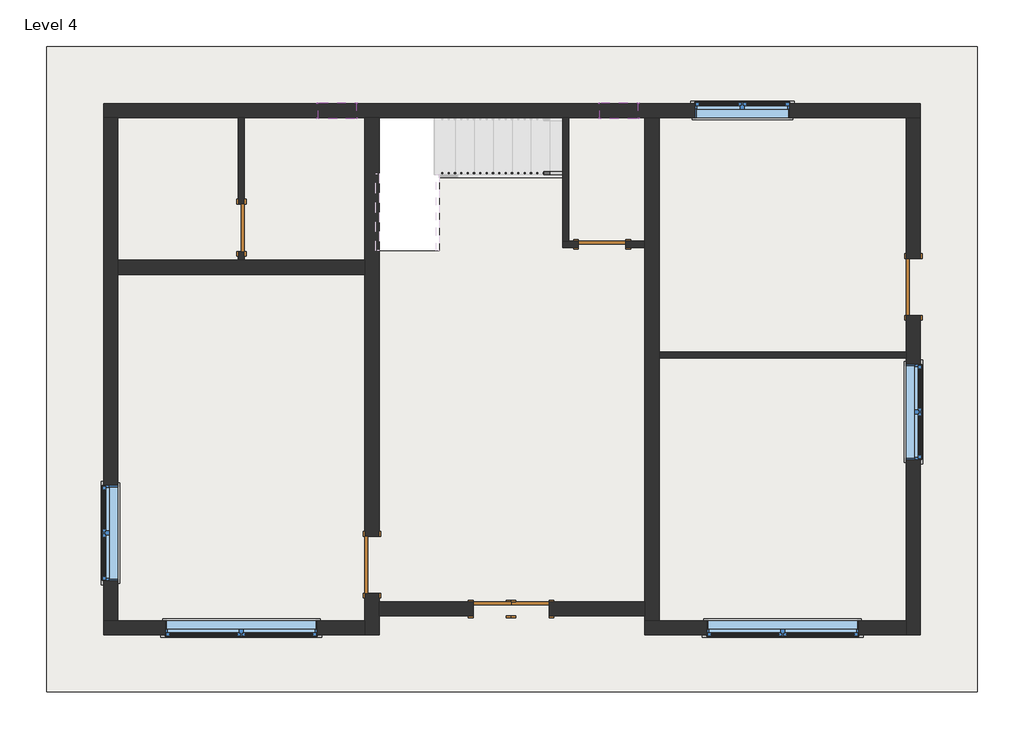
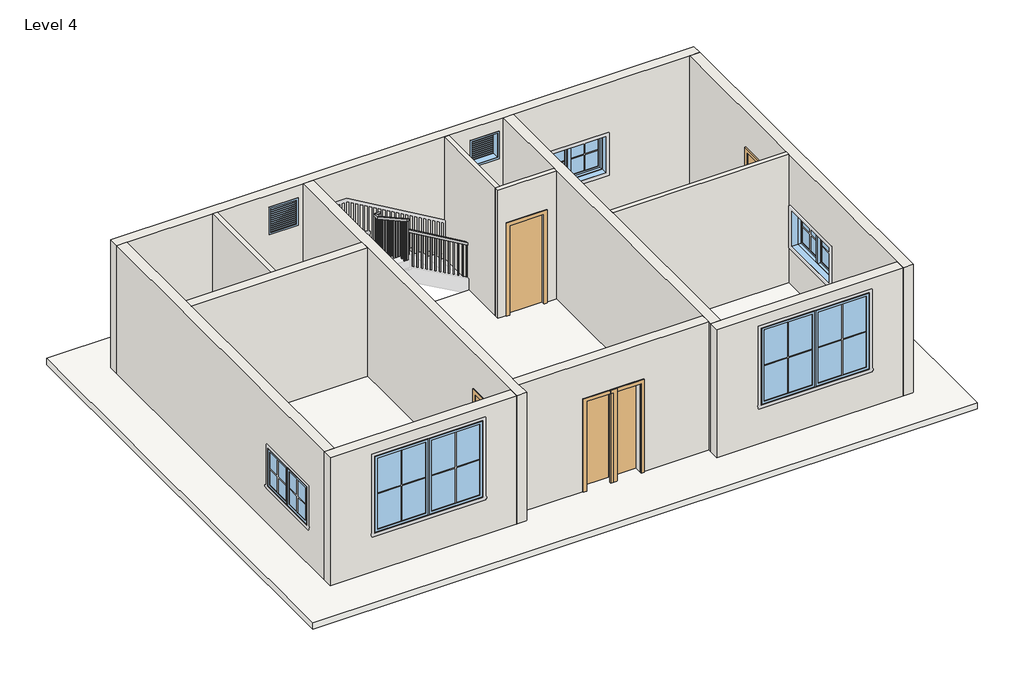
# One storey, part 1 of 2: 13 walls, 7 windows, 6 doors, 1 railing, 1 roof.
"""IFC4 building model written with IfcOpenShell, lengths in millimetres."""

from ifc_helpers import new_model, si_unit, frame, origin, place, context, project, spatial, polyline, outline, extrude, faceted_brep, transform, mapped, element, save
from components import single_flush_door_2_4a3212df, single_flush_door_2_0d3b4037, door_270f2424, door_aa9e95e7, single_flush_door_3_a90ba1ad, window_casement_double_c1d95f0f, window_casement_double_9ae172a2, window_f2d8fef0

model = new_model("IFC4")

# Units and contexts
model_context = context("Model", 3, world=origin())
ifc_project = project(units=[si_unit("LENGTHUNIT", "METRE", prefix="MILLI")], contexts=[model_context])

# Site, building, storey
site = spatial("IfcSite", under=ifc_project)
building = spatial("IfcBuilding", under=site)
storey = spatial("IfcBuildingStorey", under=building, Name="Level 4", Elevation=9448.8)

# Doors
placement = place(None, origin())
single_flush_door_2_shape = single_flush_door_2_4a3212df(model_context)
element("IfcDoor", 1, ObjectType="Single-Flush : DOOR 2'", at=placement, inside=storey, context=model_context, shape_type="MappedRepresentation", body=[
    mapped(single_flush_door_2_shape, transform((-1572.7415084, -2604.3618005, 9448.8), x_axis=(-1.0, 0.0, 0.0), y_axis=(0.0, -1.0, 0.0), z_axis=(0.0, 0.0, 1.0))),
])
single_flush_door_2_2_shape = single_flush_door_2_0d3b4037(model_context)
element("IfcDoor", 2, ObjectType="Single-Flush : DOOR 2'", at=placement, inside=storey, context=model_context, shape_type="MappedRepresentation", body=[
    mapped(single_flush_door_2_2_shape, transform((-963.1415084, -2604.3618005, 9448.8), x_axis=(1.0, 0.0, 0.0), y_axis=(0.0, 1.0, 0.0), z_axis=(0.0, 0.0, 1.0))),
])
door_shape = door_270f2424(model_context)
element("IfcDoor", 3, ObjectType="Single-Flush : DOOR 2'6\"", at=placement, inside=storey, context=model_context, shape_type="MappedRepresentation", body=[
    mapped(door_shape, transform((-5598.6415084, 3517.0381995, 9448.8), x_axis=(0.0, -1.0, 0.0), y_axis=(1.0, 0.0, 0.0), z_axis=(0.0, 0.0, 1.0))),
])
door_2_shape = door_aa9e95e7(model_context)
element("IfcDoor", 4, ObjectType="Single-Flush : DOOR 2'6\"", at=placement, inside=storey, context=model_context, shape_type="MappedRepresentation", body=[
    mapped(door_2_shape, transform((192.5584916, 3250.3381995, 9448.8), x_axis=(-1.0, 0.0, 0.0), y_axis=(0.0, -1.0, 0.0), z_axis=(0.0, 0.0, 1.0))),
])
single_flush_door_3_shape = single_flush_door_3_a90ba1ad(model_context)
element("IfcDoor", 5, ObjectType="Single-Flush : DOOR 3'", at=placement, inside=storey, context=model_context, shape_type="MappedRepresentation", body=[
    mapped(single_flush_door_3_shape, transform((-3503.1415084, -1893.1618005, 9448.8), x_axis=(0.0, -1.0, 0.0), y_axis=(1.0, 0.0, 0.0), z_axis=(0.0, 0.0, 1.0))),
])
element("IfcDoor", 6, ObjectType="Single-Flush : DOOR 3'", at=placement, inside=storey, context=model_context, shape_type="MappedRepresentation", body=[
    mapped(single_flush_door_3_shape, transform((5183.6584916, 2564.5381995, 9448.8), x_axis=(0.0, -1.0, 0.0), y_axis=(1.0, 0.0, 0.0), z_axis=(0.0, 0.0, 1.0))),
])

# Railing
element("IfcRailing", 7, ObjectType="Handrail - Rectangular", at=placement, inside=storey, context=model_context, shape_type="SolidModel", body=[
    faceted_brep([(-442.4415084, 4368.3146777, 10532.5333333), (-442.4415084, 4368.3146777, 10473.7219871), (-442.4415084, 4419.1146777, 10473.7219871), (-442.4415084, 4419.1146777, 10532.5333333), (-2398.2415084, 4368.3146777, 11673.4166667), (-2449.0415084, 4368.3146777, 11644.2386538), (-2449.0415084, 4419.1146777, 11644.2386538), (-2398.2415084, 4419.1146777, 11673.4166667), (-2398.2415084, 4368.3146777, 11929.5202697), (-2449.0415084, 4368.3146777, 11878.7202697), (-2449.0415084, 4419.1146777, 11878.7202697), (-2398.2415084, 4419.1146777, 11929.5202697), (-2474.4415084, 4368.3146777, 11929.5202697), (-2474.4415084, 4368.3146777, 11878.7202697), (-2525.2415084, 4419.1146777, 11878.7202697), (-2525.2415084, 4419.1146777, 11929.5202697), (-2474.4415084, 4292.1146777, 11929.5202697), (-2474.4415084, 4278.9546266, 11878.7202697), (-2525.2415084, 4278.9546266, 11878.7202697), (-2525.2415084, 4292.1146777, 11929.5202697), (-2474.4415084, 3148.7383287, 12564.5333333), (-2525.2415084, 3148.7383287, 12564.5333333), (-2525.2415084, 3148.7383287, 12506.42445), (-2474.4415084, 3148.7383287, 12506.42445)], [[[0, 1, 2, 3]], [[1, 0, 4, 5]], [[2, 1, 5, 6]], [[3, 2, 6, 7]], [[0, 3, 7, 4]], [[5, 4, 8, 9]], [[6, 5, 9, 10]], [[7, 6, 10, 11]], [[4, 7, 11, 8]], [[9, 8, 12, 13]], [[10, 9, 13, 14]], [[11, 10, 14, 15]], [[8, 11, 15, 12]], [[13, 12, 16, 17]], [[14, 13, 17, 18]], [[15, 14, 18, 19]], [[12, 15, 19, 16]], [[20, 21, 22, 23]], [[17, 16, 20, 23]], [[18, 17, 23, 22]], [[19, 18, 22, 21]], [[16, 19, 21, 20]]]),
    extrude(outline(polyline([(3184.0396777, 12486.9754052), (3184.0396777, 11480.8), (3164.9896777, 11480.8), (3164.9896777, 12497.5554726), (3184.0396777, 12486.9754052)])), frame((-2509.3665084, 0.0, 0.0), z_axis=(1.0, 0.0, 0.0), x_axis=(0.0, 1.0, 0.0)), (0.0, 0.0, 1.0), 19.05),
    extrude(outline(polyline([(3285.6396777, 12430.5483789), (3285.6396777, 11480.8), (3266.5896777, 11480.8), (3266.5896777, 12441.1284463), (3285.6396777, 12430.5483789)])), frame((-2509.3665084, 0.0, 0.0), z_axis=(1.0, 0.0, 0.0), x_axis=(0.0, 1.0, 0.0)), (0.0, 0.0, 1.0), 19.05),
    extrude(outline(polyline([(3387.2396777, 12374.1213526), (3387.2396777, 11480.8), (3368.1896777, 11480.8), (3368.1896777, 12384.7014201), (3387.2396777, 12374.1213526)])), frame((-2509.3665084, 0.0, 0.0), z_axis=(1.0, 0.0, 0.0), x_axis=(0.0, 1.0, 0.0)), (0.0, 0.0, 1.0), 19.05),
    extrude(outline(polyline([(3488.8396777, 12317.6420718), (3488.8396777, 11311.4666667), (3469.7896777, 11311.4666667), (3469.7896777, 12328.2221392), (3488.8396777, 12317.6420718)])), frame((-2509.3665084, 0.0, 0.0), z_axis=(1.0, 0.0, 0.0), x_axis=(0.0, 1.0, 0.0)), (0.0, 0.0, 1.0), 19.05),
    extrude(outline(polyline([(3590.4396777, 12261.2150456), (3590.4396777, 11311.4666667), (3571.3896777, 11311.4666667), (3571.3896777, 12271.795113), (3590.4396777, 12261.2150456)])), frame((-2509.3665084, 0.0, 0.0), z_axis=(1.0, 0.0, 0.0), x_axis=(0.0, 1.0, 0.0)), (0.0, 0.0, 1.0), 19.05),
    extrude(outline(polyline([(3692.0396777, 12204.7880193), (3692.0396777, 11311.4666667), (3672.9896777, 11311.4666667), (3672.9896777, 12215.3680867), (3692.0396777, 12204.7880193)])), frame((-2509.3665084, 0.0, 0.0), z_axis=(1.0, 0.0, 0.0), x_axis=(0.0, 1.0, 0.0)), (0.0, 0.0, 1.0), 19.05),
    extrude(outline(polyline([(3793.6396777, 12148.3087385), (3793.6396777, 11142.1333333), (3774.5896777, 11142.1333333), (3774.5896777, 12158.8888059), (3793.6396777, 12148.3087385)])), frame((-2509.3665084, 0.0, 0.0), z_axis=(1.0, 0.0, 0.0), x_axis=(0.0, 1.0, 0.0)), (0.0, 0.0, 1.0), 19.05),
    extrude(outline(polyline([(3895.2396777, 12091.8817122), (3895.2396777, 11142.1333333), (3876.1896777, 11142.1333333), (3876.1896777, 12102.4617797), (3895.2396777, 12091.8817122)])), frame((-2509.3665084, 0.0, 0.0), z_axis=(1.0, 0.0, 0.0), x_axis=(0.0, 1.0, 0.0)), (0.0, 0.0, 1.0), 19.05),
    extrude(outline(polyline([(3996.8396777, 12035.454686), (3996.8396777, 11142.1333333), (3977.7896777, 11142.1333333), (3977.7896777, 12046.0347534), (3996.8396777, 12035.454686)])), frame((-2509.3665084, 0.0, 0.0), z_axis=(1.0, 0.0, 0.0), x_axis=(0.0, 1.0, 0.0)), (0.0, 0.0, 1.0), 19.05),
    extrude(outline(polyline([(4098.4396777, 11978.9754052), (4098.4396777, 10972.8), (4079.3896777, 10972.8), (4079.3896777, 11989.5554726), (4098.4396777, 11978.9754052)])), frame((-2509.3665084, 0.0, 0.0), z_axis=(1.0, 0.0, 0.0), x_axis=(0.0, 1.0, 0.0)), (0.0, 0.0, 1.0), 19.05),
    extrude(outline(polyline([(4200.0396777, 11922.5483789), (4200.0396777, 10972.8), (4180.9896777, 10972.8), (4180.9896777, 11933.1284463), (4200.0396777, 11922.5483789)])), frame((-2509.3665084, 0.0, 0.0), z_axis=(1.0, 0.0, 0.0), x_axis=(0.0, 1.0, 0.0)), (0.0, 0.0, 1.0), 19.05),
    extrude(outline(polyline([(4301.6396777, 11866.1213526), (4301.6396777, 10972.8), (4282.5896777, 10972.8), (4282.5896777, 11876.7014201), (4301.6396777, 11866.1213526)])), frame((-2509.3665084, 0.0, 0.0), z_axis=(1.0, 0.0, 0.0), x_axis=(0.0, 1.0, 0.0)), (0.0, 0.0, 1.0), 19.05),
    extrude(outline(polyline([(-2464.9165084, 4384.1896777), (-2483.9665084, 4384.1896777), (-2483.9665084, 4403.2396777), (-2464.9165084, 4403.2396777), (-2464.9165084, 4384.1896777)])), frame((0.0, 0.0, 10803.4666667), z_axis=(0.0, 0.0, 1.0), x_axis=(1.0, 0.0, 0.0)), (0.0, 0.0, 1.0), 1075.253603),
    extrude(outline(polyline([(11605.3449038, -2382.3665084), (10634.1333333, -2382.3665084), (10634.1333333, -2363.3165084), (11594.2324038, -2363.3165084), (11605.3449038, -2382.3665084)])), frame((0.0, 4384.1896777, 0.0), z_axis=(0.0, 1.0, 0.0), x_axis=(0.0, 0.0, 1.0)), (0.0, 0.0, 1.0), 19.05),
    extrude(outline(polyline([(11546.0782371, -2280.7665084), (10634.1333333, -2280.7665084), (10634.1333333, -2261.7165084), (11534.9657371, -2261.7165084), (11546.0782371, -2280.7665084)])), frame((0.0, 4384.1896777, 0.0), z_axis=(0.0, 1.0, 0.0), x_axis=(0.0, 0.0, 1.0)), (0.0, 0.0, 1.0), 19.05),
    extrude(outline(polyline([(11486.8115704, -2179.1665084), (10634.1333333, -2179.1665084), (10634.1333333, -2160.1165084), (11475.6990704, -2160.1165084), (11486.8115704, -2179.1665084)])), frame((0.0, 4384.1896777, 0.0), z_axis=(0.0, 1.0, 0.0), x_axis=(0.0, 0.0, 1.0)), (0.0, 0.0, 1.0), 19.05),
    extrude(outline(polyline([(11427.5449038, -2077.5665084), (10464.8, -2077.5665084), (10464.8, -2058.5165084), (11416.4324038, -2058.5165084), (11427.5449038, -2077.5665084)])), frame((0.0, 4384.1896777, 0.0), z_axis=(0.0, 1.0, 0.0), x_axis=(0.0, 0.0, 1.0)), (0.0, 0.0, 1.0), 19.05),
    extrude(outline(polyline([(11368.2782371, -1975.9665084), (10464.8, -1975.9665084), (10464.8, -1956.9165084), (11357.1657371, -1956.9165084), (11368.2782371, -1975.9665084)])), frame((0.0, 4384.1896777, 0.0), z_axis=(0.0, 1.0, 0.0), x_axis=(0.0, 0.0, 1.0)), (0.0, 0.0, 1.0), 19.05),
    extrude(outline(polyline([(11309.0115704, -1874.3665084), (10464.8, -1874.3665084), (10464.8, -1855.3165084), (11297.8990704, -1855.3165084), (11309.0115704, -1874.3665084)])), frame((0.0, 4384.1896777, 0.0), z_axis=(0.0, 1.0, 0.0), x_axis=(0.0, 0.0, 1.0)), (0.0, 0.0, 1.0), 19.05),
    extrude(outline(polyline([(11249.7449038, -1772.7665084), (10295.4666667, -1772.7665084), (10295.4666667, -1753.7165084), (11238.6324038, -1753.7165084), (11249.7449038, -1772.7665084)])), frame((0.0, 4384.1896777, 0.0), z_axis=(0.0, 1.0, 0.0), x_axis=(0.0, 0.0, 1.0)), (0.0, 0.0, 1.0), 19.05),
    extrude(outline(polyline([(11190.4782371, -1671.1665084), (10295.4666667, -1671.1665084), (10295.4666667, -1652.1165084), (11179.3657371, -1652.1165084), (11190.4782371, -1671.1665084)])), frame((0.0, 4384.1896777, 0.0), z_axis=(0.0, 1.0, 0.0), x_axis=(0.0, 0.0, 1.0)), (0.0, 0.0, 1.0), 19.05),
    extrude(outline(polyline([(11131.2115704, -1569.5665084), (10295.4666667, -1569.5665084), (10295.4666667, -1550.5165084), (11120.0990704, -1550.5165084), (11131.2115704, -1569.5665084)])), frame((0.0, 4384.1896777, 0.0), z_axis=(0.0, 1.0, 0.0), x_axis=(0.0, 0.0, 1.0)), (0.0, 0.0, 1.0), 19.05),
    extrude(outline(polyline([(11071.9449038, -1467.9665084), (10126.1333333, -1467.9665084), (10126.1333333, -1448.9165084), (11060.8324038, -1448.9165084), (11071.9449038, -1467.9665084)])), frame((0.0, 4384.1896777, 0.0), z_axis=(0.0, 1.0, 0.0), x_axis=(0.0, 0.0, 1.0)), (0.0, 0.0, 1.0), 19.05),
    extrude(outline(polyline([(11012.6782371, -1366.3665084), (10126.1333333, -1366.3665084), (10126.1333333, -1347.3165084), (11001.5657371, -1347.3165084), (11012.6782371, -1366.3665084)])), frame((0.0, 4384.1896777, 0.0), z_axis=(0.0, 1.0, 0.0), x_axis=(0.0, 0.0, 1.0)), (0.0, 0.0, 1.0), 19.05),
    extrude(outline(polyline([(10953.4115704, -1264.7665084), (10126.1333333, -1264.7665084), (10126.1333333, -1245.7165084), (10942.2990704, -1245.7165084), (10953.4115704, -1264.7665084)])), frame((0.0, 4384.1896777, 0.0), z_axis=(0.0, 1.0, 0.0), x_axis=(0.0, 0.0, 1.0)), (0.0, 0.0, 1.0), 19.05),
    extrude(outline(polyline([(10894.1449038, -1163.1665084), (9956.8, -1163.1665084), (9956.8, -1144.1165084), (10883.0324038, -1144.1165084), (10894.1449038, -1163.1665084)])), frame((0.0, 4384.1896777, 0.0), z_axis=(0.0, 1.0, 0.0), x_axis=(0.0, 0.0, 1.0)), (0.0, 0.0, 1.0), 19.05),
    extrude(outline(polyline([(10834.8782371, -1061.5665084), (9956.8, -1061.5665084), (9956.8, -1042.5165084), (10823.7657371, -1042.5165084), (10834.8782371, -1061.5665084)])), frame((0.0, 4384.1896777, 0.0), z_axis=(0.0, 1.0, 0.0), x_axis=(0.0, 0.0, 1.0)), (0.0, 0.0, 1.0), 19.05),
    extrude(outline(polyline([(10775.6115704, -959.9665084), (9956.8, -959.9665084), (9956.8, -940.9165084), (10764.4990704, -940.9165084), (10775.6115704, -959.9665084)])), frame((0.0, 4384.1896777, 0.0), z_axis=(0.0, 1.0, 0.0), x_axis=(0.0, 0.0, 1.0)), (0.0, 0.0, 1.0), 19.05),
    extrude(outline(polyline([(10716.3449038, -858.3665084), (9787.4666667, -858.3665084), (9787.4666667, -839.3165084), (10705.2324038, -839.3165084), (10716.3449038, -858.3665084)])), frame((0.0, 4384.1896777, 0.0), z_axis=(0.0, 1.0, 0.0), x_axis=(0.0, 0.0, 1.0)), (0.0, 0.0, 1.0), 19.05),
    extrude(outline(polyline([(10657.0782371, -756.7665084), (9787.4666667, -756.7665084), (9787.4666667, -737.7165084), (10645.9657371, -737.7165084), (10657.0782371, -756.7665084)])), frame((0.0, 4384.1896777, 0.0), z_axis=(0.0, 1.0, 0.0), x_axis=(0.0, 0.0, 1.0)), (0.0, 0.0, 1.0), 19.05),
    extrude(outline(polyline([(10597.8115704, -655.1665084), (9787.4666667, -655.1665084), (9787.4666667, -636.1165084), (10586.6990704, -636.1165084), (10597.8115704, -655.1665084)])), frame((0.0, 4384.1896777, 0.0), z_axis=(0.0, 1.0, 0.0), x_axis=(0.0, 0.0, 1.0)), (0.0, 0.0, 1.0), 19.05),
    extrude(outline(polyline([(10538.5449038, -553.5665084), (9618.1333333, -553.5665084), (9618.1333333, -534.5165084), (10527.4324038, -534.5165084), (10538.5449038, -553.5665084)])), frame((0.0, 4384.1896777, 0.0), z_axis=(0.0, 1.0, 0.0), x_axis=(0.0, 0.0, 1.0)), (0.0, 0.0, 1.0), 19.05),
    extrude(outline(polyline([(-2490.3165084, 4384.1896777), (-2509.3665084, 4384.1896777), (-2509.3665084, 4403.2396777), (-2490.3165084, 4403.2396777), (-2490.3165084, 4384.1896777)])), frame((0.0, 0.0, 10803.4666667), z_axis=(0.0, 0.0, 1.0), x_axis=(1.0, 0.0, 0.0)), (0.0, 0.0, 1.0), 1075.253603),
    extrude(outline(polyline([(3167.7883287, 12495.8443826), (3167.7883287, 11480.8), (3148.7383287, 11480.8), (3148.7383287, 12506.42445), (3167.7883287, 12495.8443826)])), frame((-2509.3665084, 0.0, 0.0), z_axis=(1.0, 0.0, 0.0), x_axis=(0.0, 1.0, 0.0)), (0.0, 0.0, 1.0), 19.05),
    extrude(outline(polyline([(10484.8344871, -461.4915084), (9618.1333333, -461.4915084), (9618.1333333, -442.4415084), (10473.7219871, -442.4415084), (10484.8344871, -461.4915084)])), frame((0.0, 4384.1896777, 0.0), z_axis=(0.0, 1.0, 0.0), x_axis=(0.0, 0.0, 1.0)), (0.0, 0.0, 1.0), 19.05),
])

# Roof
element("IfcRoof", 8, ObjectType="ROOF 6\"", at=placement, inside=storey, context=model_context, shape_type="SweptSolid", body=[
    extrude(outline(polyline([(-8722.8415084, -3937.8618005), (-8722.8415084, 6425.3381995), (6212.3584916, 6425.3381995), (6212.3584916, -3937.8618005), (-8722.8415084, -3937.8618005)]), holes=[polyline([(-3439.6415084, 5333.1381995), (-3439.6415084, 3148.7383287), (-2423.6415084, 3148.7383287), (-2423.6415084, 4317.5146777), (-442.4415084, 4317.5146777), (-442.4415084, 5333.1381995), (-3439.6415084, 5333.1381995)])]), frame((0.0, 0.0, 9296.4), z_axis=(0.0, 0.0, 1.0), x_axis=(1.0, 0.0, 0.0)), (0.0, 0.0, 1.0), 152.4),
])

# Walls
element("IfcWall", 9, ObjectType="WALL 4\"", at=placement, inside=storey, context=model_context, shape_type="SweptSolid", body=[
    extrude(outline(polyline([(3136.0381995, 11582.4), (3136.0381995, 9448.8), (2996.3381995, 9448.8), (2996.3381995, 12496.8), (5282.3381995, 12496.8), (5282.3381995, 9448.8), (3898.0381995, 9448.8), (3898.0381995, 11582.4), (3136.0381995, 11582.4)])), frame((-5649.4415084, 0.0, 0.0), z_axis=(1.0, 0.0, 0.0), x_axis=(0.0, 1.0, 0.0)), (0.0, 0.0, 1.0), 101.6),
])
element("IfcWall", 10, ObjectType="WALL 4\"", at=placement, inside=storey, context=model_context, shape_type="Brep", body=[
    faceted_brep([(-188.4415084, 3301.1381995, 11582.4), (-188.4415084, 3301.1381995, 9448.8), (-340.8415084, 3301.1381995, 9448.8), (-442.4415084, 3301.1381995, 9448.8), (-442.4415084, 3301.1381995, 12496.8), (-340.8415084, 3301.1381995, 12496.8), (878.3584916, 3301.1381995, 12496.8), (878.3584916, 3301.1381995, 9448.8), (573.5584916, 3301.1381995, 9448.8), (573.5584916, 3301.1381995, 11582.4), (-442.4415084, 3199.5381995, 9448.8), (-188.4415084, 3199.5381995, 9448.8), (-188.4415084, 3199.5381995, 11582.4), (573.5584916, 3199.5381995, 11582.4), (573.5584916, 3199.5381995, 9448.8), (878.3584916, 3199.5381995, 9448.8), (878.3584916, 3199.5381995, 12496.8), (-442.4415084, 3199.5381995, 12496.8)], [[[0, 1, 2, 3, 4, 5, 6, 7, 8, 9]], [[10, 11, 12, 13, 14, 15, 16, 17]], [[8, 7, 15, 14]], [[3, 2, 1, 11, 10]], [[7, 6, 16, 15]], [[4, 3, 10, 17]], [[12, 11, 1, 0]], [[13, 12, 0, 9]], [[14, 13, 9, 8]], [[6, 5, 4, 17, 16]]]),
])
element("IfcWall", 11, ObjectType="WALL 4\"", at=placement, inside=storey, context=model_context, shape_type="Brep", body=[
    faceted_brep([(-340.8415084, 3301.1381995, 9448.8), (-340.8415084, 5282.3381995, 9448.8), (-340.8415084, 5282.3381995, 12496.8), (-340.8415084, 3301.1381995, 12496.8), (-442.4415084, 3301.1381995, 9448.8), (-442.4415084, 3301.1381995, 12496.8), (-442.4415084, 4317.5146777, 12496.8), (-442.4415084, 5282.3381995, 12496.8), (-442.4415084, 5282.3381995, 9448.8)], [[[0, 1, 2, 3]], [[4, 5, 6, 7, 8]], [[1, 0, 4, 8]], [[0, 3, 5, 4]], [[2, 1, 8, 7]], [[3, 2, 7, 6, 5]]]),
])
element("IfcWall", 12, ObjectType="WALL 4\"", at=placement, inside=storey, context=model_context, shape_type="SweptSolid", body=[
    extrude(outline(polyline([(1106.9584916, 1523.1381995), (5069.3584916, 1523.1381995), (5069.3584916, 1421.5381995), (1106.9584916, 1421.5381995), (1106.9584916, 1523.1381995)])), frame((0.0, 0.0, 9448.8), z_axis=(0.0, 0.0, 1.0), x_axis=(1.0, 0.0, 0.0)), (0.0, 0.0, 1.0), 3048.0),
])
element("IfcWall", 13, ObjectType="WALL 9\"", at=placement, inside=storey, context=model_context, shape_type="Brep", body=[
    faceted_brep([(-7808.4415084, 5282.3381995, 9448.8), (-7579.8415084, 5282.3381995, 9448.8), (-5649.4415084, 5282.3381995, 9448.8), (-5547.8415084, 5282.3381995, 9448.8), (-3617.4415084, 5282.3381995, 9448.8), (-3388.8415084, 5282.3381995, 9448.8), (-442.4415084, 5282.3381995, 9448.8), (-340.8415084, 5282.3381995, 9448.8), (878.3584916, 5282.3381995, 9448.8), (1106.9584916, 5282.3381995, 9448.8), (5069.3584916, 5282.3381995, 9448.8), (5297.9584916, 5282.3381995, 9448.8), (5297.9584916, 5282.3381995, 12496.8), (5069.3584916, 5282.3381995, 12496.8), (1106.9584916, 5282.3381995, 12496.8), (878.3584916, 5282.3381995, 12496.8), (-340.8415084, 5282.3381995, 12496.8), (-442.4415084, 5282.3381995, 12496.8), (-3388.8415084, 5282.3381995, 12496.8), (-3617.4415084, 5282.3381995, 12496.8), (-5547.8415084, 5282.3381995, 12496.8), (-5649.4415084, 5282.3381995, 12496.8), (-7579.8415084, 5282.3381995, 12496.8), (-7808.4415084, 5282.3381995, 12496.8), (3202.4584916, 5282.3381995, 11277.6), (3202.4584916, 5282.3381995, 10363.2), (1678.4584916, 5282.3381995, 10363.2), (1678.4584916, 5282.3381995, 11277.6), (154.4584916, 5282.3381995, 12192.0), (764.0584916, 5282.3381995, 12192.0), (764.0584916, 5282.3381995, 11582.4), (154.4584916, 5282.3381995, 11582.4), (-3757.1415084, 5282.3381995, 12192.0), (-3757.1415084, 5282.3381995, 11582.4), (-4366.7415084, 5282.3381995, 11582.4), (-4366.7415084, 5282.3381995, 12192.0), (-7808.4415084, 5510.9381995, 9448.8), (-7808.4415084, 5510.9381995, 12496.8), (5297.9584916, 5510.9381995, 12496.8), (5297.9584916, 5510.9381995, 9448.8), (3202.4584916, 5510.9381995, 11277.6), (1678.4584916, 5510.9381995, 11277.6), (1678.4584916, 5510.9381995, 10363.2), (3202.4584916, 5510.9381995, 10363.2), (154.4584916, 5510.9381995, 12192.0), (154.4584916, 5510.9381995, 11582.4), (764.0584916, 5510.9381995, 11582.4), (764.0584916, 5510.9381995, 12192.0), (-3757.1415084, 5510.9381995, 12192.0), (-4366.7415084, 5510.9381995, 12192.0), (-4366.7415084, 5510.9381995, 11582.4), (-3757.1415084, 5510.9381995, 11582.4)], [[[0, 1, 2, 3, 4, 5, 6, 7, 8, 9, 10, 11, 12, 13, 14, 15, 16, 17, 18, 19, 20, 21, 22, 23], [24, 25, 26, 27], [28, 29, 30, 31], [32, 33, 34, 35]], [[36, 37, 38, 39], [40, 41, 42, 43], [44, 45, 46, 47], [48, 49, 50, 51]], [[11, 10, 9, 8, 7, 6, 5, 4, 3, 2, 1, 0, 36, 39]], [[23, 22, 21, 20, 19, 18, 17, 16, 15, 14, 13, 12, 38, 37]], [[12, 11, 39, 38]], [[0, 23, 37, 36]], [[25, 24, 40, 43]], [[26, 25, 43, 42]], [[27, 26, 42, 41]], [[24, 27, 41, 40]], [[45, 44, 28, 31]], [[46, 45, 31, 30]], [[47, 46, 30, 29]], [[44, 47, 29, 28]], [[33, 32, 48, 51]], [[34, 33, 51, 50]], [[35, 34, 50, 49]], [[32, 35, 49, 48]]]),
])
element("IfcWall", 14, ObjectType="WALL 9\"", at=placement, inside=storey, context=model_context, shape_type="Brep", body=[
    faceted_brep([(5069.3584916, 2107.3381995, 11582.4), (5069.3584916, 2107.3381995, 9448.8), (5069.3584916, 1523.1381995, 9448.8), (5069.3584916, 1421.5381995, 9448.8), (5069.3584916, -2794.8618005, 9448.8), (5069.3584916, -3023.4618005, 9448.8), (5069.3584916, -3023.4618005, 12496.8), (5069.3584916, -2794.8618005, 12496.8), (5069.3584916, 1421.5381995, 12496.8), (5069.3584916, 1523.1381995, 12496.8), (5069.3584916, 5282.3381995, 12496.8), (5069.3584916, 5282.3381995, 9448.8), (5069.3584916, 3021.7381995, 9448.8), (5069.3584916, 3021.7381995, 11582.4), (5069.3584916, -204.0618005, 11277.6), (5069.3584916, -204.0618005, 10363.2), (5069.3584916, 1319.9381995, 10363.2), (5069.3584916, 1319.9381995, 11277.6), (5297.9584916, -3023.4618005, 9448.8), (5297.9584916, 2107.3381995, 9448.8), (5297.9584916, 2107.3381995, 11582.4), (5297.9584916, 3021.7381995, 11582.4), (5297.9584916, 3021.7381995, 9448.8), (5297.9584916, 5282.3381995, 9448.8), (5297.9584916, 5282.3381995, 12496.8), (5297.9584916, -3023.4618005, 12496.8), (5297.9584916, -204.0618005, 11277.6), (5297.9584916, 1319.9381995, 11277.6), (5297.9584916, 1319.9381995, 10363.2), (5297.9584916, -204.0618005, 10363.2)], [[[0, 1, 2, 3, 4, 5, 6, 7, 8, 9, 10, 11, 12, 13], [14, 15, 16, 17]], [[18, 19, 20, 21, 22, 23, 24, 25], [26, 27, 28, 29]], [[12, 11, 23, 22]], [[5, 4, 3, 2, 1, 19, 18]], [[11, 10, 24, 23]], [[6, 5, 18, 25]], [[15, 14, 26, 29]], [[16, 15, 29, 28]], [[17, 16, 28, 27]], [[14, 17, 27, 26]], [[20, 19, 1, 0]], [[21, 20, 0, 13]], [[22, 21, 13, 12]], [[10, 9, 8, 7, 6, 25, 24]]]),
])
element("IfcWall", 15, ObjectType="WALL 9\"", at=placement, inside=storey, context=model_context, shape_type="Brep", body=[
    faceted_brep([(5069.3584916, -2794.8618005, 9448.8), (1106.9584916, -2794.8618005, 9448.8), (878.3584916, -2794.8618005, 9448.8), (878.3584916, -2794.8618005, 12496.8), (1106.9584916, -2794.8618005, 12496.8), (5069.3584916, -2794.8618005, 12496.8), (1868.9584916, -2794.8618005, 12192.0), (1868.9584916, -2794.8618005, 10363.2), (4307.3584916, -2794.8618005, 10363.2), (4307.3584916, -2794.8618005, 12192.0), (5069.3584916, -3023.4618005, 9448.8), (5069.3584916, -3023.4618005, 12496.8), (878.3584916, -3023.4618005, 12496.8), (878.3584916, -3023.4618005, 9448.8), (1868.9584916, -3023.4618005, 12192.0), (4307.3584916, -3023.4618005, 12192.0), (4307.3584916, -3023.4618005, 10363.2), (1868.9584916, -3023.4618005, 10363.2)], [[[0, 1, 2, 3, 4, 5], [6, 7, 8, 9]], [[10, 11, 12, 13], [14, 15, 16, 17]], [[2, 1, 0, 10, 13]], [[0, 5, 11, 10]], [[3, 2, 13, 12]], [[7, 6, 14, 17]], [[8, 7, 17, 16]], [[9, 8, 16, 15]], [[6, 9, 15, 14]], [[5, 4, 3, 12, 11]]]),
])
element("IfcWall", 16, ObjectType="WALL 9\"", at=placement, inside=storey, context=model_context, shape_type="Brep", body=[
    faceted_brep([(1106.9584916, -2794.8618005, 9448.8), (1106.9584916, 1421.5381995, 9448.8), (1106.9584916, 1523.1381995, 9448.8), (1106.9584916, 5282.3381995, 9448.8), (1106.9584916, 5282.3381995, 12496.8), (1106.9584916, 1523.1381995, 12496.8), (1106.9584916, 1421.5381995, 12496.8), (1106.9584916, -2794.8618005, 12496.8), (878.3584916, -2794.8618005, 9448.8), (878.3584916, -2794.8618005, 12496.8), (878.3584916, -2718.6618005, 12496.8), (878.3584916, -2490.0618005, 12496.8), (878.3584916, 3199.5381995, 12496.8), (878.3584916, 3301.1381995, 12496.8), (878.3584916, 5282.3381995, 12496.8), (878.3584916, 5282.3381995, 9448.8), (878.3584916, 3301.1381995, 9448.8), (878.3584916, 3199.5381995, 9448.8), (878.3584916, -2490.0618005, 9448.8), (878.3584916, -2718.6618005, 9448.8)], [[[0, 1, 2, 3, 4, 5, 6, 7]], [[8, 9, 10, 11, 12, 13, 14, 15, 16, 17, 18, 19]], [[3, 2, 1, 0, 8, 19, 18, 17, 16, 15]], [[0, 7, 9, 8]], [[4, 3, 15, 14]], [[7, 6, 5, 4, 14, 13, 12, 11, 10, 9]]]),
])
element("IfcWall", 17, ObjectType="WALL 9\"", at=placement, inside=storey, context=model_context, shape_type="SweptSolid", body=[
    extrude(outline(polyline([(9448.8, 878.3584916), (12496.8, 878.3584916), (12496.8, -3388.8415084), (9448.8, -3388.8415084), (9448.8, -1877.5415084), (11582.4, -1877.5415084), (11582.4, -658.3415084), (9448.8, -658.3415084), (9448.8, 878.3584916)])), frame((0.0, -2718.6618005, 0.0), z_axis=(0.0, 1.0, 0.0), x_axis=(0.0, 0.0, 1.0)), (0.0, 0.0, 1.0), 228.6),
])
element("IfcWall", 18, ObjectType="WALL 9\"", at=placement, inside=storey, context=model_context, shape_type="Brep", body=[
    faceted_brep([(-3388.8415084, -3023.4618005, 9448.8), (-3388.8415084, -2718.6618005, 9448.8), (-3388.8415084, -2490.0618005, 9448.8), (-3388.8415084, -2350.3618005, 9448.8), (-3388.8415084, -2350.3618005, 11582.4), (-3388.8415084, -1435.9618005, 11582.4), (-3388.8415084, -1435.9618005, 9448.8), (-3388.8415084, 5282.3381995, 9448.8), (-3388.8415084, 5282.3381995, 12496.8), (-3388.8415084, -2490.0618005, 12496.8), (-3388.8415084, -2718.6618005, 12496.8), (-3388.8415084, -3023.4618005, 12496.8), (-3617.4415084, -2350.3618005, 11582.4), (-3617.4415084, -2350.3618005, 9448.8), (-3617.4415084, -2794.8618005, 9448.8), (-3617.4415084, -3023.4618005, 9448.8), (-3617.4415084, -3023.4618005, 12496.8), (-3617.4415084, -2794.8618005, 12496.8), (-3617.4415084, 2767.7381995, 12496.8), (-3617.4415084, 2996.3381995, 12496.8), (-3617.4415084, 5282.3381995, 12496.8), (-3617.4415084, 5282.3381995, 9448.8), (-3617.4415084, 2996.3381995, 9448.8), (-3617.4415084, 2767.7381995, 9448.8), (-3617.4415084, -1435.9618005, 9448.8), (-3617.4415084, -1435.9618005, 11582.4)], [[[0, 1, 2, 3, 4, 5, 6, 7, 8, 9, 10, 11]], [[12, 13, 14, 15, 16, 17, 18, 19, 20, 21, 22, 23, 24, 25]], [[15, 14, 13, 3, 2, 1, 0]], [[24, 23, 22, 21, 7, 6]], [[11, 10, 9, 8, 20, 19, 18, 17, 16]], [[8, 7, 21, 20]], [[0, 11, 16, 15]], [[4, 3, 13, 12]], [[5, 4, 12, 25]], [[6, 5, 25, 24]]]),
])
element("IfcWall", 19, ObjectType="WALL 9\"", at=placement, inside=storey, context=model_context, shape_type="Brep", body=[
    faceted_brep([(-3617.4415084, -2794.8618005, 9448.8), (-7579.8415084, -2794.8618005, 9448.8), (-7808.4415084, -2794.8618005, 9448.8), (-7808.4415084, -2794.8618005, 12496.8), (-7579.8415084, -2794.8618005, 12496.8), (-3617.4415084, -2794.8618005, 12496.8), (-6817.8415084, -2794.8618005, 12192.0), (-6817.8415084, -2794.8618005, 10363.2), (-4379.4415084, -2794.8618005, 10363.2), (-4379.4415084, -2794.8618005, 12192.0), (-3617.4415084, -3023.4618005, 9448.8), (-3617.4415084, -3023.4618005, 12496.8), (-7808.4415084, -3023.4618005, 12496.8), (-7808.4415084, -3023.4618005, 9448.8), (-6817.8415084, -3023.4618005, 12192.0), (-4379.4415084, -3023.4618005, 12192.0), (-4379.4415084, -3023.4618005, 10363.2), (-6817.8415084, -3023.4618005, 10363.2)], [[[0, 1, 2, 3, 4, 5], [6, 7, 8, 9]], [[10, 11, 12, 13], [14, 15, 16, 17]], [[2, 1, 0, 10, 13]], [[0, 5, 11, 10]], [[3, 2, 13, 12]], [[7, 6, 14, 17]], [[8, 7, 17, 16]], [[9, 8, 16, 15]], [[6, 9, 15, 14]], [[5, 4, 3, 12, 11]]]),
])
element("IfcWall", 20, ObjectType="WALL 9\"", at=placement, inside=storey, context=model_context, shape_type="Brep", body=[
    faceted_brep([(-7579.8415084, -2794.8618005, 9448.8), (-7579.8415084, 2767.7381995, 9448.8), (-7579.8415084, 2996.3381995, 9448.8), (-7579.8415084, 5282.3381995, 9448.8), (-7579.8415084, 5282.3381995, 12496.8), (-7579.8415084, 2996.3381995, 12496.8), (-7579.8415084, 2767.7381995, 12496.8), (-7579.8415084, -2794.8618005, 12496.8), (-7579.8415084, -623.1618005, 11277.6), (-7579.8415084, -623.1618005, 10363.2), (-7579.8415084, -2147.1618005, 10363.2), (-7579.8415084, -2147.1618005, 11277.6), (-7808.4415084, -2794.8618005, 9448.8), (-7808.4415084, -2794.8618005, 12496.8), (-7808.4415084, 5282.3381995, 12496.8), (-7808.4415084, 5282.3381995, 9448.8), (-7808.4415084, -623.1618005, 11277.6), (-7808.4415084, -2147.1618005, 11277.6), (-7808.4415084, -2147.1618005, 10363.2), (-7808.4415084, -623.1618005, 10363.2)], [[[0, 1, 2, 3, 4, 5, 6, 7], [8, 9, 10, 11]], [[12, 13, 14, 15], [16, 17, 18, 19]], [[3, 2, 1, 0, 12, 15]], [[0, 7, 13, 12]], [[4, 3, 15, 14]], [[9, 8, 16, 19]], [[10, 9, 19, 18]], [[11, 10, 18, 17]], [[8, 11, 17, 16]], [[7, 6, 5, 4, 14, 13]]]),
])
element("IfcWall", 21, ObjectType="WALL 9\"", at=placement, inside=storey, context=model_context, shape_type="Brep", body=[
    faceted_brep([(-7579.8415084, 2767.7381995, 9448.8), (-3617.4415084, 2767.7381995, 9448.8), (-3617.4415084, 2767.7381995, 12496.8), (-7579.8415084, 2767.7381995, 12496.8), (-7579.8415084, 2996.3381995, 9448.8), (-7579.8415084, 2996.3381995, 12496.8), (-5649.4415084, 2996.3381995, 12496.8), (-5547.8415084, 2996.3381995, 12496.8), (-3617.4415084, 2996.3381995, 12496.8), (-3617.4415084, 2996.3381995, 9448.8), (-5547.8415084, 2996.3381995, 9448.8), (-5649.4415084, 2996.3381995, 9448.8)], [[[0, 1, 2, 3]], [[4, 5, 6, 7, 8, 9, 10, 11]], [[1, 0, 4, 11, 10, 9]], [[2, 1, 9, 8]], [[0, 3, 5, 4]], [[3, 2, 8, 7, 6, 5]]]),
])

# Windows
window_casement_double_shape = window_casement_double_c1d95f0f(model_context)
element("IfcWindow", 22, ObjectType="Window-Casement-Double", at=placement, inside=storey, context=model_context, shape_type="MappedRepresentation", body=[
    mapped(window_casement_double_shape, transform((-7694.1415084, -1385.1618005, 9448.8), x_axis=(0.0, 1.0, 0.0), y_axis=(-1.0, 0.0, 0.0), z_axis=(0.0, 0.0, 1.0))),
])
element("IfcWindow", 23, ObjectType="Window-Casement-Double", at=placement, inside=storey, context=model_context, shape_type="MappedRepresentation", body=[
    mapped(window_casement_double_shape, transform((5183.6584916, 557.9381995, 9448.8), x_axis=(0.0, -1.0, 0.0), y_axis=(1.0, 0.0, 0.0), z_axis=(0.0, 0.0, 1.0))),
])
element("IfcWindow", 24, ObjectType="Window-Casement-Double", at=placement, inside=storey, context=model_context, shape_type="MappedRepresentation", body=[
    mapped(window_casement_double_shape, transform((2440.4584916, 5396.6381995, 9448.8), x_axis=(1.0, 0.0, 0.0), y_axis=(0.0, 1.0, 0.0), z_axis=(0.0, 0.0, 1.0))),
])
window_casement_double_2_shape = window_casement_double_9ae172a2(model_context)
element("IfcWindow", 25, ObjectType="Window-Casement-Double", at=placement, inside=storey, context=model_context, shape_type="MappedRepresentation", body=[
    mapped(window_casement_double_2_shape, transform((-5598.6415084, -2909.1618005, 9448.8), x_axis=(-1.0, 0.0, 0.0), y_axis=(0.0, -1.0, 0.0), z_axis=(0.0, 0.0, 1.0))),
])
element("IfcWindow", 26, ObjectType="Window-Casement-Double", at=placement, inside=storey, context=model_context, shape_type="MappedRepresentation", body=[
    mapped(window_casement_double_2_shape, transform((3088.1584916, -2909.1618005, 9448.8), x_axis=(-1.0, 0.0, 0.0), y_axis=(0.0, -1.0, 0.0), z_axis=(0.0, 0.0, 1.0))),
])
window_shape = window_f2d8fef0(model_context)
element("IfcWindow", 27, ObjectType="Window-Louvers : 24\" x 24\"", at=placement, inside=storey, context=model_context, shape_type="MappedRepresentation", body=[
    mapped(window_shape, transform((459.2584916, 5402.9881995, 10668.0), x_axis=(1.0, 0.0, 0.0), y_axis=(0.0, 1.0, 0.0), z_axis=(0.0, 0.0, 1.0))),
])
element("IfcWindow", 28, ObjectType="Window-Louvers : 24\" x 24\"", at=placement, inside=storey, context=model_context, shape_type="MappedRepresentation", body=[
    mapped(window_shape, transform((-4061.9415084, 5390.2881995, 10668.0), x_axis=(-1.0, 0.0, 0.0), y_axis=(0.0, -1.0, 0.0), z_axis=(0.0, 0.0, 1.0))),
])

save(model, "model.ifc")

# Revit data of these elements
# Type "Single-Flush : DOOR 2'"
#   Type Mark = "10"
#   Construction Type Id = "MDOOR"
#   Assembly Code = "C1020"
#   Analytic Construction = "Metal"
#   Thickness = 0' - 2"
#   Heat Transfer Coefficient (U) = 0.651978 BTU/(h·ft²·°F)
#   Height = 7' - 0"
#   Trim Projection Ext = 0' - 1"
#   Trim Projection Int = 0' - 1"
#   Trim Width = 0' - 3"
#   Width = 2' - 0"
#   Define Thermal Properties by = 1
#   Door Material = Door - Panel
#   Frame Material = Door - Frame
#   Visual Light Transmittance = 0
#   Solar Heat Gain Coefficient = 0
#   Function = (empty or 0)
#   Wall Closure = (empty or 0)
# Type "Single-Flush : DOOR 2'6\""
#   Type Mark = "9"
#   Construction Type Id = "MDOOR"
#   Assembly Code = "C1020"
#   Analytic Construction = "Metal"
#   Thickness = 0' - 2"
#   Heat Transfer Coefficient (U) = 0.651978 BTU/(h·ft²·°F)
#   Height = 7' - 0"
#   Trim Projection Ext = 0' - 1"
#   Trim Projection Int = 0' - 1"
#   Trim Width = 0' - 3"
#   Width = 2' - 6"
#   Define Thermal Properties by = 1
#   Door Material = Door - Panel
#   Frame Material = Door - Frame
#   Visual Light Transmittance = 0
#   Solar Heat Gain Coefficient = 0
#   Function = (empty or 0)
#   Wall Closure = (empty or 0)
# Type "Single-Flush : DOOR 3'"
#   Type Mark = "8"
#   Construction Type Id = "MDOOR"
#   Assembly Code = "C1020"
#   Analytic Construction = "Metal"
#   Thickness = 0' - 2"
#   Heat Transfer Coefficient (U) = 0.651978 BTU/(h·ft²·°F)
#   Height = 7' - 0"
#   Trim Projection Ext = 0' - 1"
#   Trim Projection Int = 0' - 1"
#   Trim Width = 0' - 3"
#   Width = 3' - 0"
#   Define Thermal Properties by = 1
#   Door Material = Door - Panel
#   Frame Material = Door - Frame
#   Visual Light Transmittance = 0
#   Solar Heat Gain Coefficient = 0
#   Function = (empty or 0)
#   Wall Closure = (empty or 0)
# Type "Handrail - Rectangular"
#   Assembly Code = "C2010400"
#   built-in parameter 1008612 = 0.0416667 (stored number, unit not read)
#   built-in parameter 1008611 = 0.0416667 (stored number, unit not read)
#   built-in parameter 1008609 = 0.333333 (stored number, unit not read)
#   built-in parameter 1008604 = 0.166667 (stored number, unit not read)
#   built-in parameter 1008603 = 0.166667 (stored number, unit not read)
#   Railing Height = 3' - 0"
#   built-in parameter 1008630 = 2
#   built-in parameter 1008610 = 2
#   built-in parameter 1008618 = Baluster - Square : 3/4"
# Type "ROOF 6\""
#   Assembly Code = "B1020"
#   Layers, outside or top first: 0' - 6" no material (function 1)
# Type "WALL 4\""
#   Assembly Code = "B2010"
#   Layers, outside or top first: 0' - 4" no material (function 1)
# Type "WALL 9\""
#   Assembly Code = "B2010"
#   Layers, outside or top first: 0' - 9" no material (function 1)
# Type "Window-Casement-Double"
#   Type Mark = "18"
#   Fire Rating = "0.5h"
#   Assembly Code = "B2020100"
#   Analytic Construction = "Double glazing - domestic"
#   Frame Extension [instance default] = 0' - 0 1/4"
#   Window Inset [instance default] = 0' - 0"
#   Wall Thickness [instance default] = 0' - 6"
#   Interior Wall Closure [instance default] = 0' - 2 1/4"
#   Half Width = 2' - 6"
#   Visual Light Transmittance = 0.81
#   Thermal Resistance (R) = 1.8146 (h·ft²·°F)/BTU
#   Solar Heat Gain Coefficient = 0.76
#   Rough Width = 5' - 0 1/2"
#   Rough Height = 3' - 0 1/2"
#   Height = 3' - 0"
#   Heat Transfer Coefficient (U) = 0.5511 BTU/(h·ft²·°F)
#   Exterior Wall Closure [instance default] = 0' - 1 1/4"
#   Extension Jamb [instance default] = 0' - 2 1/4"
#   Default Sill Height = 3' - 0"
#   Width = 5' - 0"
#   Muntin Visibility = yes
#   Interior Trim Visibility [instance default] = yes
#   Exterior Trim Visibility [instance default] = yes
#   Extension Jamb Visibility [instance default] = yes
#   Interior Trim Material = Wood - Stained
#   Muntin Pattern = Muntin Pattern_2x2 : Muntin Pattern_2x2
#   Interior Trim = Trim-Window-Interior-Flat : Picture Frame
#   Interior Frame Material = Wood - Stained
#   Glass Panel Material = Glass
#   Exterior Trim Material = Clad - White
#   Exterior Trim = Trim-Window-Exterior-Flat : with Sill
#   Exterior Frame Material = Clad - White
#   Wall Closure = (empty or 0)
# Type "Window-Casement-Double"
#   Type Mark = "19"
#   Fire Rating = "0.5h"
#   Assembly Code = "B2020100"
#   Analytic Construction = "Double glazing - domestic"
#   Frame Extension [instance default] = 0' - 0 1/4"
#   Window Inset [instance default] = 0' - 0"
#   Wall Thickness [instance default] = 0' - 6"
#   Interior Wall Closure [instance default] = 0' - 2 1/4"
#   Half Width = 4' - 0"
#   Visual Light Transmittance = 0.81
#   Thermal Resistance (R) = 1.8146 (h·ft²·°F)/BTU
#   Solar Heat Gain Coefficient = 0.76
#   Rough Width = 8' - 0 1/2"
#   Rough Height = 6' - 0 1/2"
#   Height = 6' - 0"
#   Heat Transfer Coefficient (U) = 0.5511 BTU/(h·ft²·°F)
#   Exterior Wall Closure [instance default] = 0' - 1 1/4"
#   Extension Jamb [instance default] = 0' - 2 1/4"
#   Default Sill Height = 3' - 0"
#   Width = 8' - 0"
#   Muntin Visibility = yes
#   Interior Trim Visibility [instance default] = yes
#   Exterior Trim Visibility [instance default] = yes
#   Extension Jamb Visibility [instance default] = yes
#   Interior Trim Material = Wood - Stained
#   Muntin Pattern = Muntin Pattern_2x2 : Muntin Pattern_2x2
#   Interior Trim = Trim-Window-Interior-Flat : Picture Frame
#   Interior Frame Material = Wood - Stained
#   Glass Panel Material = Glass
#   Exterior Trim Material = Clad - White
#   Exterior Trim = Trim-Window-Exterior-Flat : with Sill
#   Exterior Frame Material = Clad - White
#   Wall Closure = (empty or 0)
# Type "Window-Louvers : 24\" x 24\""
#   Type Mark = "20"
#   Construction Type Id = "GSP4R"
#   Assembly Code = "B20"
#   Analytic Construction = "1/8 in Pilkington single glazing"
#   Visual Light Transmittance = 0.9
#   Thermal Resistance (R) = 1.53941 (h·ft²·°F)/BTU
#   Solar Heat Gain Coefficient = 0.78
#   Max Height = 1' - 11.74264"
#   Height = 2' - 0"
#   Heat Transfer Coefficient (U) = 0.6496 BTU/(h·ft²·°F)
#   Blade Width [instance default] = 1' - 10 1/2"
#   Blade Vertical Thickness = 0' - 0.35355"
#   Blade Thickness = 0' - 0 1/4"
#   Blade Spacing = 0' - 1 1/2"
#   Blade Height = 0' - 1.85355"
#   Blade Depth = 0' - 3"
#   Blade Angle = 45.00°
#   Default Sill Height = 3' - 0"
#   Trim Projection_Exterior = 0' - 0 1/2"
#   Trim Projection_Interior = 0' - 0 1/2"
#   Trim Width_Exterior = 0' - 1 1/2"
#   Trim Width_Interior = 0' - 1 1/2"
#   Width = 2' - 0"
#   Max Blade Count = 12
#   Define Thermal Properties by = 1
#   Blade Count = 12
#   Frame Material = Birch
#   Louver Material = Birch
#   Trim Exterior Material = Birch
#   Trim Interior Material = Birch
#   Wall Closure = (empty or 0)
# Elements 1, 2 (IfcDoor, "Single-Flush : DOOR 2'")
#   Phase Created = New Construction
#   Materials on its faces: "Door - Frame", "Door - Panel"
# Elements 3, 4 (IfcDoor, "Single-Flush : DOOR 2'6\"")
#   Phase Created = New Construction
#   Materials on its faces: "Door - Frame", "Door - Panel"
# Elements 5, 6 (IfcDoor, "Single-Flush : DOOR 3'")
#   Phase Created = New Construction
#   Materials on its faces: "Door - Frame", "Door - Panel"
# Element 7 (IfcRailing, "Handrail - Rectangular")
#   Phase Created = New Construction
# Element 8 (IfcRoof, "ROOF 6\"")
#   built-in parameter 1001705 = 31 (stored number, unit not read)
#   built-in parameter 1001701 = -0.5 (stored number, unit not read)
#   built-in parameter 1001710 = 33615
#   Phase Created = New Construction
#   Materials on its faces: "Door - Frame", "Default Roof", "Wood - Stained"
# Elements 9, 12 (IfcWall, "WALL 4\"")
#   Top Offset = 0' - 0"
#   Base Offset = 0' - 0"
#   Unconnected Height = 10' - 0"
#   wall height = 10' - 0"
#   Phase Created = New Construction
#   Base Constraint = Level 4
#   Materials on its faces: "Default Wall"
# Elements 10, 11 (IfcWall, "WALL 4\"")
#   Top Offset = 0' - 0"
#   Base Offset = 0' - 0"
#   Unconnected Height = 10' - 0"
#   wall height = 10' - 0"
#   Phase Created = New Construction
#   Base Constraint = Level 4
#   Materials on its faces: "Default Wall", "Door - Frame"
# Element 13 (IfcWall, "WALL 9\"")
#   Top Offset = 0' - 0"
#   Base Offset = 0' - 0"
#   Unconnected Height = 10' - 0"
#   wall height = 10' - 0"
#   Phase Created = New Construction
#   Base Constraint = Level 4
#   Materials on its faces: "Default Wall", "Parking Stripe", "Door - Frame"
# Elements 14, 15, 16, 17, 19, 20 (IfcWall, "WALL 9\"")
#   Top Offset = 0' - 0"
#   Base Offset = 0' - 0"
#   Unconnected Height = 10' - 0"
#   wall height = 10' - 0"
#   Phase Created = New Construction
#   Base Constraint = Level 4
#   Materials on its faces: "Default Wall", "Parking Stripe"
# Element 18 (IfcWall, "WALL 9\"")
#   Top Offset = 0' - 0"
#   Base Offset = 0' - 0"
#   Unconnected Height = 10' - 0"
#   wall height = 10' - 0"
#   Phase Created = New Construction
#   Base Constraint = Level 4
#   Materials on its faces: "Default Wall", "Door - Frame", "Parking Stripe"
# Element 21 (IfcWall, "WALL 9\"")
#   Top Offset = 0' - 0"
#   Base Offset = 0' - 0"
#   Unconnected Height = 10' - 0"
#   wall height = 10' - 0"
#   Phase Created = New Construction
#   Base Constraint = Level 4
#   Materials on its faces: "Default Wall"
# Element 22 (IfcWindow, "Window-Casement-Double")
#   Mark = "22"
#   Window Inset = 0' - 0"
#   Interior Wall Closure = 0' - 2 1/4"
#   Frame Extension = 0' - 0 1/4"
#   Exterior Wall Closure = 0' - 1 1/4"
#   Interior Trim Visibility = yes
#   Exterior Trim Visibility = yes
#   Phase Created = New Construction
#   Materials on its faces: "Wood - Stained", "Glass", "Clad - White"
# Element 23 (IfcWindow, "Window-Casement-Double")
#   Mark = "23"
#   Window Inset = 0' - 0"
#   Interior Wall Closure = 0' - 2 1/4"
#   Frame Extension = 0' - 0 1/4"
#   Exterior Wall Closure = 0' - 1 1/4"
#   Interior Trim Visibility = yes
#   Exterior Trim Visibility = yes
#   Phase Created = New Construction
#   Materials on its faces: "Wood - Stained", "Glass", "Clad - White"
# Element 24 (IfcWindow, "Window-Casement-Double")
#   Mark = "24"
#   Window Inset = 0' - 0"
#   Interior Wall Closure = 0' - 2 1/4"
#   Frame Extension = 0' - 0 1/4"
#   Exterior Wall Closure = 0' - 1 1/4"
#   Interior Trim Visibility = yes
#   Exterior Trim Visibility = yes
#   Phase Created = New Construction
#   Materials on its faces: "Wood - Stained", "Glass", "Clad - White"
# Element 25 (IfcWindow, "Window-Casement-Double")
#   Mark = "25"
#   Window Inset = 0' - 0"
#   Interior Wall Closure = 0' - 2 1/4"
#   Frame Extension = 0' - 0 1/4"
#   Exterior Wall Closure = 0' - 1 1/4"
#   Interior Trim Visibility = yes
#   Exterior Trim Visibility = yes
#   Phase Created = New Construction
#   Materials on its faces: "Wood - Stained", "Glass", "Clad - White"
# Element 26 (IfcWindow, "Window-Casement-Double")
#   Mark = "26"
#   Window Inset = 0' - 0"
#   Interior Wall Closure = 0' - 2 1/4"
#   Frame Extension = 0' - 0 1/4"
#   Exterior Wall Closure = 0' - 1 1/4"
#   Interior Trim Visibility = yes
#   Exterior Trim Visibility = yes
#   Phase Created = New Construction
#   Materials on its faces: "Wood - Stained", "Glass", "Clad - White"
# Element 27 (IfcWindow, "Window-Louvers : 24\" x 24\"")
#   Mark = "27"
#   Blade Width = 1' - 10 1/2"
#   Phase Created = New Construction
#   Materials on its faces: "Birch"
# Element 28 (IfcWindow, "Window-Louvers : 24\" x 24\"")
#   Mark = "28"
#   Blade Width = 1' - 10 1/2"
#   Phase Created = New Construction
#   Materials on its faces: "Birch"
# Materials
#   "Door - Panel": class "Wood", colour RGB 210 159 95, transparency 0, Cost = 0
#   "Door - Frame": colour RGB 118 70 51, transparency 0, Cost = 0
#   "Wood - Stained": class "Wood", colour RGB 224 178 126, transparency 0, Cost = 0
#   "Glass": class "Glass", colour RGB 0 128 192, transparency 0.75, Description = "Soda Lime Glass", Cost = 0
#   "Clad - White": class "Wood", colour RGB 242 242 238, transparency 0, Cost = 0
#   "Birch": class "Wood", colour RGB 224 178 126, transparency 0, Description = "Betula Alleghaniensis", Cost = 0
#   "Default Roof": colour RGB 88 101 114, transparency 0, Cost = 0
#   "Default Wall": colour RGB 128 128 128, transparency 0, Cost = 0
#   "Parking Stripe": class "Paint", colour RGB 250 250 91, transparency 0, Cost = 0
